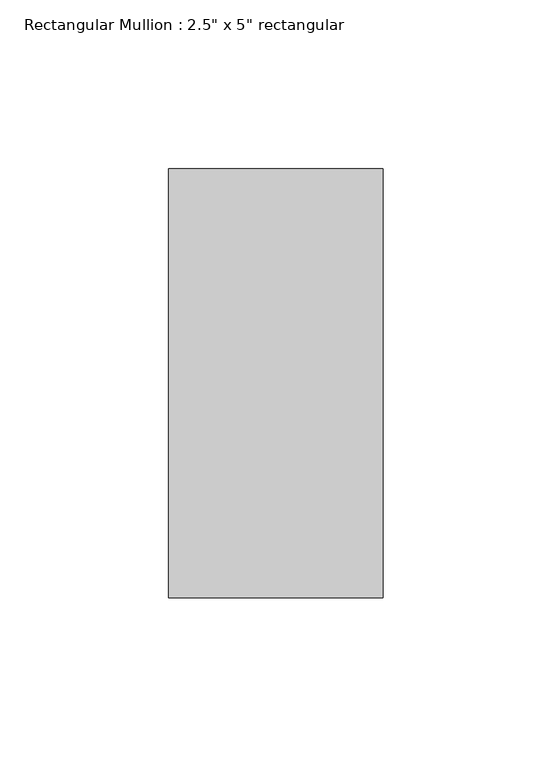
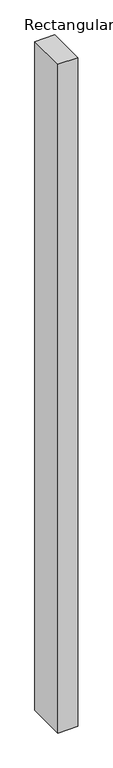
"""IFC4 building model written with IfcOpenShell, lengths in millimetres: member geometry."""

from ifc_helpers import new_model, si_unit, frame, origin, place, context, project, spatial, polyline, outline, extrude, source, transform, mapped, element, save


def member_c3d994c2(model_context):
    return source(origin(), model_context, "Body", "SweptSolid", [
        extrude(outline(polyline([(0.0, 63.5), (0.0, -63.5), (-63.5, -63.5), (-63.5, 63.5), (0.0, 63.5)])), frame((0.0, 0.0, -2254.3645985), z_axis=(0.0, 0.0, 1.0), x_axis=(1.0, 0.0, 0.0)), (0.0, 0.0, 1.0), 2254.3645985),
    ])


if __name__ == "__main__":
    model = new_model("IFC4")
    model_context = context("Model", 3, world=origin())
    ifc_project = project(units=[si_unit("LENGTHUNIT", "METRE", prefix="MILLI")], contexts=[model_context])
    site = spatial("IfcSite", under=ifc_project)
    building = spatial("IfcBuilding", under=site)
    placement = place(None, origin())
    member_shape = member_c3d994c2(model_context)
    element("IfcMember", 1, ObjectType="Rectangular Mullion : 2.5\" x 5\" rectangular", at=placement, inside=building, context=model_context, shape_type="MappedRepresentation", body=[
        mapped(member_shape, transform((0.0, 0.0, 0.0), x_axis=(1.0, 0.0, 0.0), y_axis=(0.0, 1.0, 0.0), z_axis=(0.0, 0.0, 1.0))),
    ])
    save(model, "model.ifc")

# Revit data of these elements
# Type "Rectangular Mullion : 2.5\" x 5\" rectangular"
#   built-in parameter 1007304 = 0.416667 (stored number, unit not read)
#   built-in parameter 1007301 = 0.104167 (stored number, unit not read)
#   built-in parameter 1007300 = 0.104167 (stored number, unit not read)
# Element 1 (IfcMember, "Rectangular Mullion : 2.5\" x 5\" rectangular")
#   Materials on its faces: "Aluminum"
# Materials
#   "Aluminum": class "Metal", colour RGB 247 247 247, transparency 0, Description = "Aluminum 6061", Cost = 0
